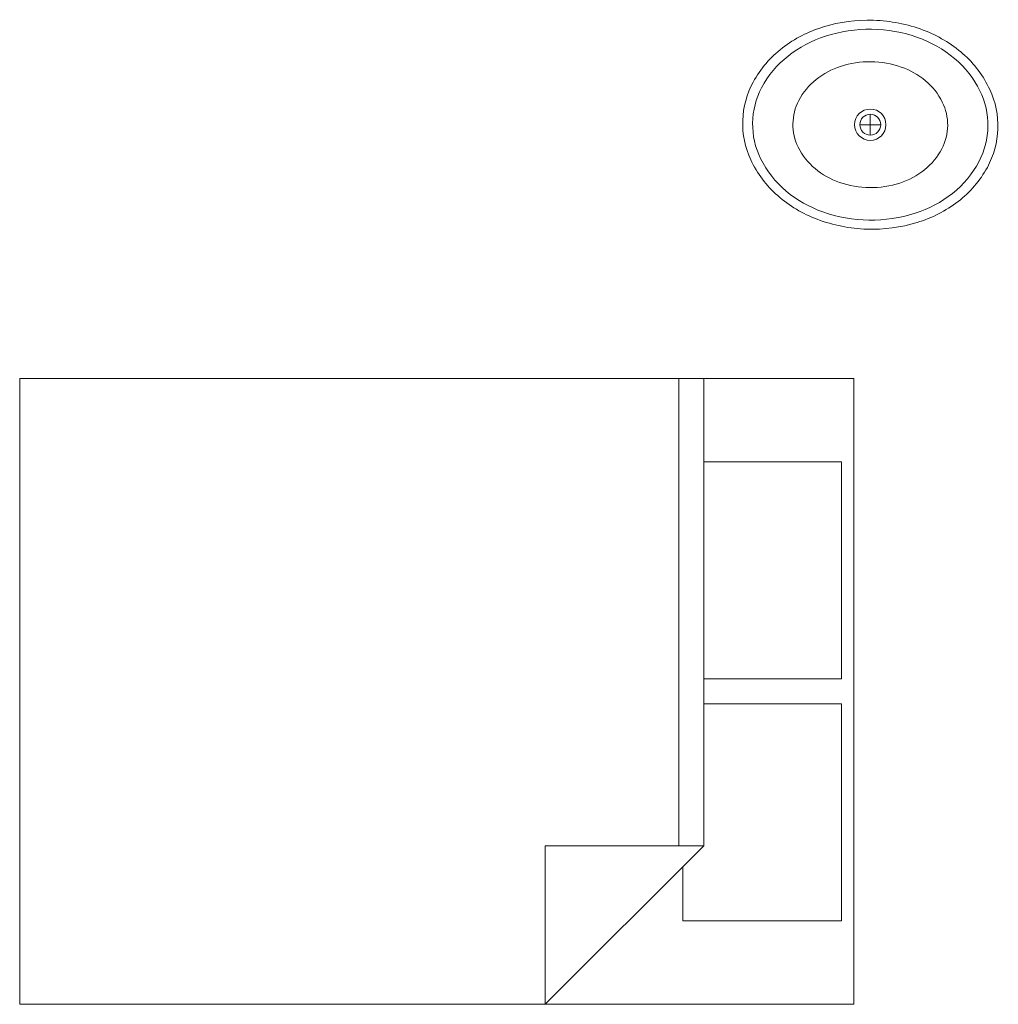
# Model space of a CAD drawing. Units: inches. Extents: x -977 to 1065, y -406 to 125.
# Tile 1 of 4: x -977 to -883, y -268 to -174. Entities that reach past the tile are written whole.
import ezdxf

# ---------------------------------------------------------------- set-up
doc = ezdxf.new("R2010")
doc.units = ezdxf.units.IN
doc.header["$MEASUREMENT"] = 0
doc.layers.add('A-FLOR-FIXT', color=8, linetype='Continuous', lineweight=18)
doc.layers.add('A-FURN', color=8, linetype='Continuous', lineweight=18)

# ---------------------------------------------------------------- blocks, each defined once
blk = doc.blocks.new('Sink - Oval top')
for p, q in [((0, 1), (0, -1)), ((-1, 0), (1, 0))]:
    blk.add_line(p, q)
for points in [[(-12.234, 0.394, 0.117634), (-11.465, -3.362, 0.104469), (-8.879, -6.804, 0.090016), (-5.083, -9.072, 0.08192), (-0.323, -10.016, 0.08192), (4.488, -9.381, 0.090016), (8.422, -7.361, 0.104469), (11.224, -4.093, 0.117634), (12.234, -0.394, 0.117634), (11.465, 3.362, 0.104469), (8.879, 6.804, 0.090016), (5.083, 9.072, 0.08192), (0.323, 10.016, 0.08192), (-4.488, 9.381, 0.090016), (-8.422, 7.361, 0.104469), (-11.224, 4.093, 0.117634)], [(-11.286, 0.159, 0.118622), (-10.516, -3.253, 0.104678), (-8.072, -6.359, 0.089562), (-4.538, -8.367, 0.081185), (-0.129, -9.152, 0.081185), (4.3, -8.492, 0.089562), (7.889, -6.584, 0.104678), (10.42, -3.548, 0.118622), (11.286, -0.159, 0.118622), (10.516, 3.253, 0.104678), (8.072, 6.359, 0.089562), (4.538, 8.367, 0.081185), (0.129, 9.152, 0.081185), (-4.3, 8.492, 0.089562), (-7.889, 6.584, 0.104678), (-10.42, 3.548, 0.118622)], [(-7.42, 0.083, 0.118283), (-6.907, -2.167, 0.104607), (-5.295, -4.21, 0.089718), (-2.967, -5.528, 0.081436), (-0.068, -6.037, 0.081436), (2.842, -5.593, 0.089718), (5.199, -4.327, 0.104607), (6.857, -2.321, 0.118283), (7.42, -0.083, 0.118283), (6.907, 2.167, 0.104607), (5.295, 4.21, 0.089718), (2.967, 5.528, 0.081436), (0.068, 6.037, 0.081436), (-2.842, 5.593, 0.089718), (-5.199, 4.327, 0.104607), (-6.857, 2.321, 0.118283)]]:
    blk.add_lwpolyline(points, format="xyb", close=True)
for radius in [1.5, 1]:
    blk.add_circle((0, 0), radius)
blk = doc.blocks.new('Bed - Queen')
for p, q in [((0, -80.00003), (0, 0)), ((0, 0), (59.99999, 0)), ((59.99999, 0), (59.99999, -80.00003)), ((7.99999, -1.2), (28.79998, -1.2)), ((7.99999, -14.4), (7.99999, -1.2)), ((28.79998, -1.2), (28.79998, -14.4)), ((31.19999, -1.2), (51.99999, -1.2)), ((31.19999, -14.4), (31.19999, -1.2)), ((51.99999, -1.2), (51.99999, -16.4)), ((0, -14.4), (44.8, -14.4)), ((59.99999, -29.6), (44.8, -14.4)), ((44.8, -14.4), (44.8, -29.6)), ((44.8, -16.8), (0, -16.8)), ((51.99999, -16.4), (46.79936, -16.4)), ((44.8, -29.6), (59.99999, -29.6)), ((59.99999, -80.00003), (0, -80.00003))]:
    blk.add_line(p, q)

msp = doc.modelspace()

# ---------------------------------------------------------------- block references
at = {"layer": 'A-FLOR-FIXT'}
msp.add_blockref('Sink - Oval top', (-895.423, -184.025), dxfattribs=at)
at = {"layer": 'A-FURN', "rotation": 270}
msp.add_blockref('Bed - Queen', (-896.99, -208.366), dxfattribs=at)

doc.saveas('drawing.dxf')
